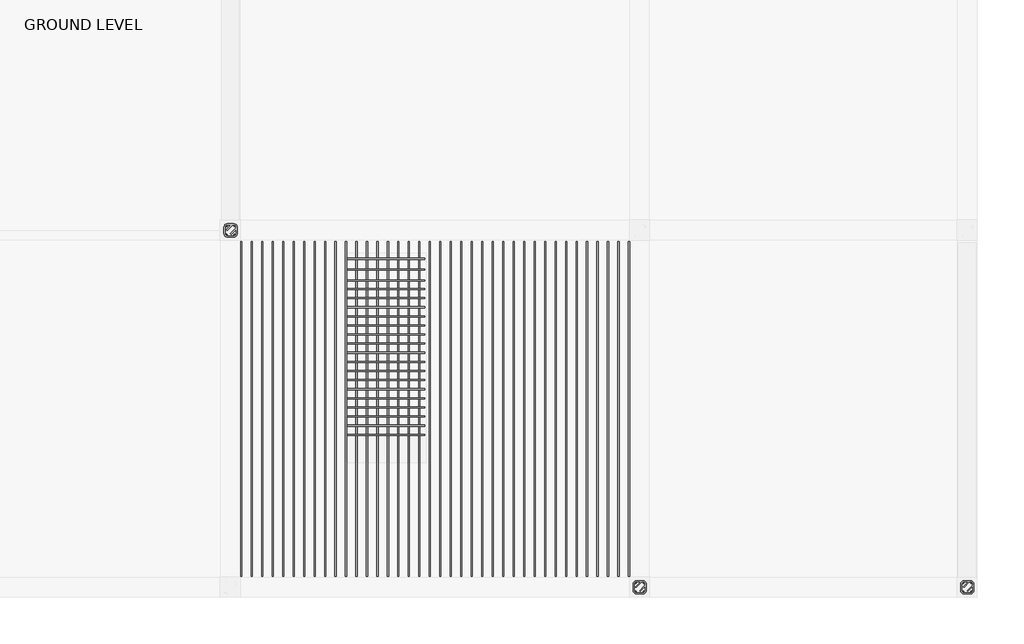
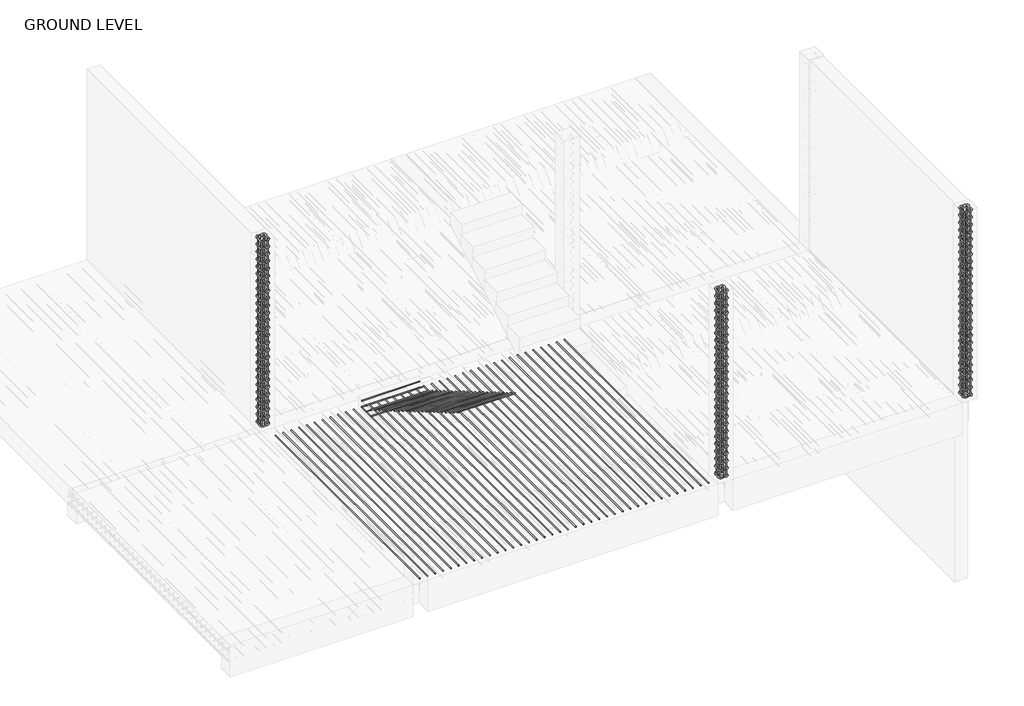
# One storey, part 4 of 8: 13 reinforcing bars.
"""IFC4 building model written with IfcOpenShell, lengths in millimetres."""

from ifc_helpers import new_model, si_unit, point, frame, origin, place, context, project, spatial, polyline, circle_curve, trimmed, segment, composite_curve, source, transform, mapped, element, save
from ifc_brep_helpers import swept_disk

model = new_model("IFC4")

# Units and contexts
model_context = context("Model", 3, world=origin())
ifc_project = project(units=[si_unit("LENGTHUNIT", "METRE", prefix="MILLI")], contexts=[model_context])

# Site, building, storey
site = spatial("IfcSite", under=ifc_project)
building = spatial("IfcBuilding", under=site)
storey = spatial("IfcBuildingStorey", under=building, Name="GROUND LEVEL", Elevation=0.0)

# Reinforcing bars
placement = place(None, origin())
reinforcing_bar_shape = source(origin(), model_context, "Body", "SolidModel", [
    swept_disk(composite_curve([segment(polyline([(-7435.1173382, -4134.0810507, -120.830741), (-7435.1173382, -358.1289151, -120.830741)]), True, "CONTINUOUS")], self_intersect=False), 6.35),
])
element("IfcReinforcingBar", 1, at=placement, inside=storey, context=model_context, shape_type="MappedRepresentation", body=[
    mapped(reinforcing_bar_shape, transform((0.0, 0.0, 0.0), x_axis=(1.0, 0.0, 0.0), y_axis=(0.0, 1.0, 0.0), z_axis=(0.0, 0.0, 1.0))),
    mapped(reinforcing_bar_shape, transform((-118.1294146, 0.0, 0.0), x_axis=(1.0, 0.0, 0.0), y_axis=(0.0, 1.0, 0.0), z_axis=(0.0, 0.0, 1.0))),
    mapped(reinforcing_bar_shape, transform((-236.2588293, 0.0, 0.0), x_axis=(1.0, 0.0, 0.0), y_axis=(0.0, 1.0, 0.0), z_axis=(0.0, 0.0, 1.0))),
    mapped(reinforcing_bar_shape, transform((-354.3882439, 0.0, 0.0), x_axis=(1.0, 0.0, 0.0), y_axis=(0.0, 1.0, 0.0), z_axis=(0.0, 0.0, 1.0))),
    mapped(reinforcing_bar_shape, transform((-472.5176586, 0.0, 0.0), x_axis=(1.0, 0.0, 0.0), y_axis=(0.0, 1.0, 0.0), z_axis=(0.0, 0.0, 1.0))),
    mapped(reinforcing_bar_shape, transform((-590.6470732, 0.0, 0.0), x_axis=(1.0, 0.0, 0.0), y_axis=(0.0, 1.0, 0.0), z_axis=(0.0, 0.0, 1.0))),
    mapped(reinforcing_bar_shape, transform((-708.7764878, 0.0, 0.0), x_axis=(1.0, 0.0, 0.0), y_axis=(0.0, 1.0, 0.0), z_axis=(0.0, 0.0, 1.0))),
    mapped(reinforcing_bar_shape, transform((-826.9059025, 0.0, 0.0), x_axis=(1.0, 0.0, 0.0), y_axis=(0.0, 1.0, 0.0), z_axis=(0.0, 0.0, 1.0))),
    mapped(reinforcing_bar_shape, transform((-945.0353171, 0.0, 0.0), x_axis=(1.0, 0.0, 0.0), y_axis=(0.0, 1.0, 0.0), z_axis=(0.0, 0.0, 1.0))),
    mapped(reinforcing_bar_shape, transform((-1063.1647318, 0.0, 0.0), x_axis=(1.0, 0.0, 0.0), y_axis=(0.0, 1.0, 0.0), z_axis=(0.0, 0.0, 1.0))),
    mapped(reinforcing_bar_shape, transform((-1181.2941464, 0.0, 0.0), x_axis=(1.0, 0.0, 0.0), y_axis=(0.0, 1.0, 0.0), z_axis=(0.0, 0.0, 1.0))),
    mapped(reinforcing_bar_shape, transform((-1299.423561, 0.0, 0.0), x_axis=(1.0, 0.0, 0.0), y_axis=(0.0, 1.0, 0.0), z_axis=(0.0, 0.0, 1.0))),
    mapped(reinforcing_bar_shape, transform((-1417.5529757, 0.0, 0.0), x_axis=(1.0, 0.0, 0.0), y_axis=(0.0, 1.0, 0.0), z_axis=(0.0, 0.0, 1.0))),
    mapped(reinforcing_bar_shape, transform((-1535.6823903, 0.0, 0.0), x_axis=(1.0, 0.0, 0.0), y_axis=(0.0, 1.0, 0.0), z_axis=(0.0, 0.0, 1.0))),
    mapped(reinforcing_bar_shape, transform((-1653.811805, 0.0, 0.0), x_axis=(1.0, 0.0, 0.0), y_axis=(0.0, 1.0, 0.0), z_axis=(0.0, 0.0, 1.0))),
    mapped(reinforcing_bar_shape, transform((-1771.9412196, 0.0, 0.0), x_axis=(1.0, 0.0, 0.0), y_axis=(0.0, 1.0, 0.0), z_axis=(0.0, 0.0, 1.0))),
    mapped(reinforcing_bar_shape, transform((-1890.0706342, 0.0, 0.0), x_axis=(1.0, 0.0, 0.0), y_axis=(0.0, 1.0, 0.0), z_axis=(0.0, 0.0, 1.0))),
    mapped(reinforcing_bar_shape, transform((-2008.2000489, 0.0, 0.0), x_axis=(1.0, 0.0, 0.0), y_axis=(0.0, 1.0, 0.0), z_axis=(0.0, 0.0, 1.0))),
    mapped(reinforcing_bar_shape, transform((-2126.3294635, 0.0, 0.0), x_axis=(1.0, 0.0, 0.0), y_axis=(0.0, 1.0, 0.0), z_axis=(0.0, 0.0, 1.0))),
    mapped(reinforcing_bar_shape, transform((-2244.4588782, 0.0, 0.0), x_axis=(1.0, 0.0, 0.0), y_axis=(0.0, 1.0, 0.0), z_axis=(0.0, 0.0, 1.0))),
    mapped(reinforcing_bar_shape, transform((-2362.5882928, 0.0, 0.0), x_axis=(1.0, 0.0, 0.0), y_axis=(0.0, 1.0, 0.0), z_axis=(0.0, 0.0, 1.0))),
    mapped(reinforcing_bar_shape, transform((-2480.7177075, 0.0, 0.0), x_axis=(1.0, 0.0, 0.0), y_axis=(0.0, 1.0, 0.0), z_axis=(0.0, 0.0, 1.0))),
    mapped(reinforcing_bar_shape, transform((-2598.8471221, 0.0, 0.0), x_axis=(1.0, 0.0, 0.0), y_axis=(0.0, 1.0, 0.0), z_axis=(0.0, 0.0, 1.0))),
    mapped(reinforcing_bar_shape, transform((-2716.9765367, 0.0, 0.0), x_axis=(1.0, 0.0, 0.0), y_axis=(0.0, 1.0, 0.0), z_axis=(0.0, 0.0, 1.0))),
    mapped(reinforcing_bar_shape, transform((-2835.1059514, 0.0, 0.0), x_axis=(1.0, 0.0, 0.0), y_axis=(0.0, 1.0, 0.0), z_axis=(0.0, 0.0, 1.0))),
    mapped(reinforcing_bar_shape, transform((-2953.235366, 0.0, 0.0), x_axis=(1.0, 0.0, 0.0), y_axis=(0.0, 1.0, 0.0), z_axis=(0.0, 0.0, 1.0))),
    mapped(reinforcing_bar_shape, transform((-3071.3647807, 0.0, 0.0), x_axis=(1.0, 0.0, 0.0), y_axis=(0.0, 1.0, 0.0), z_axis=(0.0, 0.0, 1.0))),
    mapped(reinforcing_bar_shape, transform((-3189.4941953, 0.0, 0.0), x_axis=(1.0, 0.0, 0.0), y_axis=(0.0, 1.0, 0.0), z_axis=(0.0, 0.0, 1.0))),
    mapped(reinforcing_bar_shape, transform((-3307.6236099, 0.0, 0.0), x_axis=(1.0, 0.0, 0.0), y_axis=(0.0, 1.0, 0.0), z_axis=(0.0, 0.0, 1.0))),
    mapped(reinforcing_bar_shape, transform((-3425.7530246, 0.0, 0.0), x_axis=(1.0, 0.0, 0.0), y_axis=(0.0, 1.0, 0.0), z_axis=(0.0, 0.0, 1.0))),
    mapped(reinforcing_bar_shape, transform((-3543.8824392, 0.0, 0.0), x_axis=(1.0, 0.0, 0.0), y_axis=(0.0, 1.0, 0.0), z_axis=(0.0, 0.0, 1.0))),
    mapped(reinforcing_bar_shape, transform((-3662.0118539, 0.0, 0.0), x_axis=(1.0, 0.0, 0.0), y_axis=(0.0, 1.0, 0.0), z_axis=(0.0, 0.0, 1.0))),
    mapped(reinforcing_bar_shape, transform((-3780.1412685, 0.0, 0.0), x_axis=(1.0, 0.0, 0.0), y_axis=(0.0, 1.0, 0.0), z_axis=(0.0, 0.0, 1.0))),
    mapped(reinforcing_bar_shape, transform((-3898.2706831, 0.0, 0.0), x_axis=(1.0, 0.0, 0.0), y_axis=(0.0, 1.0, 0.0), z_axis=(0.0, 0.0, 1.0))),
    mapped(reinforcing_bar_shape, transform((-4016.4000978, 0.0, 0.0), x_axis=(1.0, 0.0, 0.0), y_axis=(0.0, 1.0, 0.0), z_axis=(0.0, 0.0, 1.0))),
    mapped(reinforcing_bar_shape, transform((-4134.5295124, 0.0, 0.0), x_axis=(1.0, 0.0, 0.0), y_axis=(0.0, 1.0, 0.0), z_axis=(0.0, 0.0, 1.0))),
    mapped(reinforcing_bar_shape, transform((-4252.6589271, 0.0, 0.0), x_axis=(1.0, 0.0, 0.0), y_axis=(0.0, 1.0, 0.0), z_axis=(0.0, 0.0, 1.0))),
    mapped(reinforcing_bar_shape, transform((-4370.7883417, 0.0, 0.0), x_axis=(1.0, 0.0, 0.0), y_axis=(0.0, 1.0, 0.0), z_axis=(0.0, 0.0, 1.0))),
])
reinforcing_bar_2_shape = source(origin(), model_context, "Body", "SolidModel", [
    swept_disk(composite_curve([segment(polyline([(-7269.7123519, -4211.1006392, 3008.0), (-7269.7123519, -4211.1006392, 40.0)]), True, "CONTINUOUS")], self_intersect=False), 6.35),
])
element("IfcReinforcingBar", 2, at=placement, inside=storey, context=model_context, shape_type="MappedRepresentation", body=[
    mapped(reinforcing_bar_2_shape, transform((0.0, 0.0, 0.0), x_axis=(1.0, 0.0, 0.0), y_axis=(0.0, 1.0, 0.0), z_axis=(0.0, 0.0, 1.0))),
    mapped(reinforcing_bar_2_shape, transform((0.0, -96.9916148, 0.0), x_axis=(1.0, 0.0, 0.0), y_axis=(0.0, 1.0, 0.0), z_axis=(0.0, 0.0, 1.0))),
])
reinforcing_bar_3_shape = source(origin(), model_context, "Body", "SolidModel", [
    swept_disk(composite_curve([segment(polyline([(-7355.7786987, -4256.8741003, 3001.65), (-7300.0351358, -4201.1305373, 3001.65)]), True, "CONTINUOUS"), segment(trimmed(circle_curve(frame((-7277.8673382, -4223.2983349, 3001.65), z_axis=(0.0, 0.0, -1.0), x_axis=(-22.167797600000085, 22.167797600000085, 0.0)), 31.35), [point((-7300.0351358, -4201.1305373, 3001.65))], [point((-7246.5173382, -4223.2983349, 3001.65))], True, "CARTESIAN"), True, "CONTINUOUS"), segment(polyline([(-7246.5173382, -4223.2983349, 3001.65), (-7246.5173382, -4296.4983349, 3001.65)]), True, "CONTINUOUS"), segment(trimmed(circle_curve(frame((-7277.8673382, -4296.4983349, 3001.65), z_axis=(0.0, 0.0, -1.0), x_axis=(31.349999999999454, 0.0, 0.0)), 31.35), [point((-7246.5173382, -4296.4983349, 3001.65))], [point((-7277.8673382, -4327.8483349, 3001.65))], True, "CARTESIAN"), True, "CONTINUOUS"), segment(polyline([(-7277.8673382, -4327.8483349, 3001.65), (-7351.0673382, -4327.8483349, 3001.65)]), True, "CONTINUOUS"), segment(trimmed(circle_curve(frame((-7351.0673382, -4296.6343361, 3004.5669815), z_axis=(0.0, 0.09304566152621355, -0.9956618426308951), x_axis=(0.0, -31.2139987999999, -2.91698150000002)), 31.35), [point((-7351.0673382, -4327.8483349, 3001.65))], [point((-7382.4173382, -4296.6343361, 3004.5669815))], True, "CARTESIAN"), True, "CONTINUOUS"), segment(polyline([(-7382.4173382, -4296.6343361, 3004.5669815), (-7382.4173382, -4223.1623337, 3011.4330185)]), True, "CONTINUOUS"), segment(trimmed(circle_curve(frame((-7351.0673382, -4223.1623337, 3011.4330185), z_axis=(0.0, 0.09304566152621355, -0.9956618426308951), x_axis=(-31.349999999999454, 0.0, 0.0)), 31.35), [point((-7382.4173382, -4223.1623337, 3011.4330185))], [point((-7351.0673382, -4191.9483349, 3014.35))], True, "CARTESIAN"), True, "CONTINUOUS"), segment(polyline([(-7351.0673382, -4191.9483349, 3014.35), (-7277.8673382, -4191.9483349, 3014.35)]), True, "CONTINUOUS"), segment(trimmed(circle_curve(frame((-7277.8673382, -4223.2983349, 3014.35), z_axis=(0.0, 0.0, -1.0), x_axis=(0.0, 31.349999999999454, 0.0)), 31.35), [point((-7277.8673382, -4191.9483349, 3014.35))], [point((-7255.6995406, -4245.4661325, 3014.35))], True, "CARTESIAN"), True, "CONTINUOUS"), segment(polyline([(-7255.6995406, -4245.4661325, 3014.35), (-7311.4431035, -4301.2096954, 3014.35)]), True, "CONTINUOUS")], self_intersect=False), 6.35),
])
element("IfcReinforcingBar", 3, at=placement, inside=storey, context=model_context, shape_type="MappedRepresentation", body=[
    mapped(reinforcing_bar_3_shape, transform((0.0, 0.0, 0.0), x_axis=(1.0, 0.0, 0.0), y_axis=(0.0, 1.0, 0.0), z_axis=(0.0, 0.0, 1.0))),
    mapped(reinforcing_bar_3_shape, transform((0.0, 0.0, -118.212), x_axis=(1.0, 0.0, 0.0), y_axis=(0.0, 1.0, 0.0), z_axis=(0.0, 0.0, 1.0))),
    mapped(reinforcing_bar_3_shape, transform((0.0, 0.0, -236.424), x_axis=(1.0, 0.0, 0.0), y_axis=(0.0, 1.0, 0.0), z_axis=(0.0, 0.0, 1.0))),
    mapped(reinforcing_bar_3_shape, transform((0.0, 0.0, -354.636), x_axis=(1.0, 0.0, 0.0), y_axis=(0.0, 1.0, 0.0), z_axis=(0.0, 0.0, 1.0))),
    mapped(reinforcing_bar_3_shape, transform((0.0, 0.0, -472.848), x_axis=(1.0, 0.0, 0.0), y_axis=(0.0, 1.0, 0.0), z_axis=(0.0, 0.0, 1.0))),
    mapped(reinforcing_bar_3_shape, transform((0.0, 0.0, -591.06), x_axis=(1.0, 0.0, 0.0), y_axis=(0.0, 1.0, 0.0), z_axis=(0.0, 0.0, 1.0))),
    mapped(reinforcing_bar_3_shape, transform((0.0, 0.0, -709.272), x_axis=(1.0, 0.0, 0.0), y_axis=(0.0, 1.0, 0.0), z_axis=(0.0, 0.0, 1.0))),
    mapped(reinforcing_bar_3_shape, transform((0.0, 0.0, -827.484), x_axis=(1.0, 0.0, 0.0), y_axis=(0.0, 1.0, 0.0), z_axis=(0.0, 0.0, 1.0))),
    mapped(reinforcing_bar_3_shape, transform((0.0, 0.0, -945.696), x_axis=(1.0, 0.0, 0.0), y_axis=(0.0, 1.0, 0.0), z_axis=(0.0, 0.0, 1.0))),
    mapped(reinforcing_bar_3_shape, transform((0.0, 0.0, -1063.908), x_axis=(1.0, 0.0, 0.0), y_axis=(0.0, 1.0, 0.0), z_axis=(0.0, 0.0, 1.0))),
    mapped(reinforcing_bar_3_shape, transform((0.0, 0.0, -1182.12), x_axis=(1.0, 0.0, 0.0), y_axis=(0.0, 1.0, 0.0), z_axis=(0.0, 0.0, 1.0))),
    mapped(reinforcing_bar_3_shape, transform((0.0, 0.0, -1300.332), x_axis=(1.0, 0.0, 0.0), y_axis=(0.0, 1.0, 0.0), z_axis=(0.0, 0.0, 1.0))),
    mapped(reinforcing_bar_3_shape, transform((0.0, 0.0, -1418.544), x_axis=(1.0, 0.0, 0.0), y_axis=(0.0, 1.0, 0.0), z_axis=(0.0, 0.0, 1.0))),
    mapped(reinforcing_bar_3_shape, transform((0.0, 0.0, -1536.756), x_axis=(1.0, 0.0, 0.0), y_axis=(0.0, 1.0, 0.0), z_axis=(0.0, 0.0, 1.0))),
    mapped(reinforcing_bar_3_shape, transform((0.0, 0.0, -1654.968), x_axis=(1.0, 0.0, 0.0), y_axis=(0.0, 1.0, 0.0), z_axis=(0.0, 0.0, 1.0))),
    mapped(reinforcing_bar_3_shape, transform((0.0, 0.0, -1773.18), x_axis=(1.0, 0.0, 0.0), y_axis=(0.0, 1.0, 0.0), z_axis=(0.0, 0.0, 1.0))),
    mapped(reinforcing_bar_3_shape, transform((0.0, 0.0, -1891.392), x_axis=(1.0, 0.0, 0.0), y_axis=(0.0, 1.0, 0.0), z_axis=(0.0, 0.0, 1.0))),
    mapped(reinforcing_bar_3_shape, transform((0.0, 0.0, -2009.604), x_axis=(1.0, 0.0, 0.0), y_axis=(0.0, 1.0, 0.0), z_axis=(0.0, 0.0, 1.0))),
    mapped(reinforcing_bar_3_shape, transform((0.0, 0.0, -2127.816), x_axis=(1.0, 0.0, 0.0), y_axis=(0.0, 1.0, 0.0), z_axis=(0.0, 0.0, 1.0))),
    mapped(reinforcing_bar_3_shape, transform((0.0, 0.0, -2246.028), x_axis=(1.0, 0.0, 0.0), y_axis=(0.0, 1.0, 0.0), z_axis=(0.0, 0.0, 1.0))),
    mapped(reinforcing_bar_3_shape, transform((0.0, 0.0, -2364.24), x_axis=(1.0, 0.0, 0.0), y_axis=(0.0, 1.0, 0.0), z_axis=(0.0, 0.0, 1.0))),
    mapped(reinforcing_bar_3_shape, transform((0.0, 0.0, -2482.452), x_axis=(1.0, 0.0, 0.0), y_axis=(0.0, 1.0, 0.0), z_axis=(0.0, 0.0, 1.0))),
    mapped(reinforcing_bar_3_shape, transform((0.0, 0.0, -2600.664), x_axis=(1.0, 0.0, 0.0), y_axis=(0.0, 1.0, 0.0), z_axis=(0.0, 0.0, 1.0))),
    mapped(reinforcing_bar_3_shape, transform((0.0, 0.0, -2718.876), x_axis=(1.0, 0.0, 0.0), y_axis=(0.0, 1.0, 0.0), z_axis=(0.0, 0.0, 1.0))),
    mapped(reinforcing_bar_3_shape, transform((0.0, 0.0, -2837.088), x_axis=(1.0, 0.0, 0.0), y_axis=(0.0, 1.0, 0.0), z_axis=(0.0, 0.0, 1.0))),
    mapped(reinforcing_bar_3_shape, transform((0.0, 0.0, -2955.3), x_axis=(1.0, 0.0, 0.0), y_axis=(0.0, 1.0, 0.0), z_axis=(0.0, 0.0, 1.0))),
])
reinforcing_bar_4_shape = source(origin(), model_context, "Body", "SolidModel", [
    swept_disk(composite_curve([segment(polyline([(-7359.2223245, -4211.1006392, 3008.0), (-7359.2223245, -4211.1006392, 40.0)]), True, "CONTINUOUS")], self_intersect=False), 6.35),
])
element("IfcReinforcingBar", 4, at=placement, inside=storey, context=model_context, shape_type="MappedRepresentation", body=[
    mapped(reinforcing_bar_4_shape, transform((0.0, 0.0, 0.0), x_axis=(1.0, 0.0, 0.0), y_axis=(0.0, 1.0, 0.0), z_axis=(0.0, 0.0, 1.0))),
    mapped(reinforcing_bar_4_shape, transform((0.0, -96.9916148, 0.0), x_axis=(1.0, 0.0, 0.0), y_axis=(0.0, 1.0, 0.0), z_axis=(0.0, 0.0, 1.0))),
])
reinforcing_bar_5_shape = source(origin(), model_context, "Body", "SolidModel", [
    swept_disk(composite_curve([segment(polyline([(-3576.0006936, -4211.1006392, 3008.0), (-3576.0006936, -4211.1006392, 40.0)]), True, "CONTINUOUS")], self_intersect=False), 6.35),
])
element("IfcReinforcingBar", 5, at=placement, inside=storey, context=model_context, shape_type="MappedRepresentation", body=[
    mapped(reinforcing_bar_5_shape, transform((0.0, 0.0, 0.0), x_axis=(1.0, 0.0, 0.0), y_axis=(0.0, 1.0, 0.0), z_axis=(0.0, 0.0, 1.0))),
    mapped(reinforcing_bar_5_shape, transform((0.0, -96.9916148, 0.0), x_axis=(1.0, 0.0, 0.0), y_axis=(0.0, 1.0, 0.0), z_axis=(0.0, 0.0, 1.0))),
])
reinforcing_bar_6_shape = source(origin(), model_context, "Body", "SolidModel", [
    swept_disk(composite_curve([segment(polyline([(-3662.0670404, -4256.8741003, 3001.65), (-3606.3234775, -4201.1305373, 3001.65)]), True, "CONTINUOUS"), segment(trimmed(circle_curve(frame((-3584.1556799, -4223.2983349, 3001.65), z_axis=(0.0, 0.0, -1.0), x_axis=(-22.167797600000085, 22.167797600000085, 0.0)), 31.35), [point((-3606.3234775, -4201.1305373, 3001.65))], [point((-3552.8056799, -4223.2983349, 3001.65))], True, "CARTESIAN"), True, "CONTINUOUS"), segment(polyline([(-3552.8056799, -4223.2983349, 3001.65), (-3552.8056799, -4296.4983349, 3001.65)]), True, "CONTINUOUS"), segment(trimmed(circle_curve(frame((-3584.1556799, -4296.4983349, 3001.65), z_axis=(0.0, 0.0, -1.0), x_axis=(31.34999999999991, 0.0, 0.0)), 31.35), [point((-3552.8056799, -4296.4983349, 3001.65))], [point((-3584.1556799, -4327.8483349, 3001.65))], True, "CARTESIAN"), True, "CONTINUOUS"), segment(polyline([(-3584.1556799, -4327.8483349, 3001.65), (-3657.3556799, -4327.8483349, 3001.65)]), True, "CONTINUOUS"), segment(trimmed(circle_curve(frame((-3657.3556799, -4296.6343361, 3004.5669815), z_axis=(0.0, 0.09304566152621355, -0.9956618426308951), x_axis=(0.0, -31.2139987999999, -2.91698150000002)), 31.35), [point((-3657.3556799, -4327.8483349, 3001.65))], [point((-3688.7056799, -4296.6343361, 3004.5669815))], True, "CARTESIAN"), True, "CONTINUOUS"), segment(polyline([(-3688.7056799, -4296.6343361, 3004.5669815), (-3688.7056799, -4223.1623337, 3011.4330185)]), True, "CONTINUOUS"), segment(trimmed(circle_curve(frame((-3657.3556799, -4223.1623337, 3011.4330185), z_axis=(0.0, 0.09304566152621355, -0.9956618426308951), x_axis=(-31.350000000000364, 0.0, 0.0)), 31.35), [point((-3688.7056799, -4223.1623337, 3011.4330185))], [point((-3657.3556799, -4191.9483349, 3014.35))], True, "CARTESIAN"), True, "CONTINUOUS"), segment(polyline([(-3657.3556799, -4191.9483349, 3014.35), (-3584.1556799, -4191.9483349, 3014.35)]), True, "CONTINUOUS"), segment(trimmed(circle_curve(frame((-3584.1556799, -4223.2983349, 3014.35), z_axis=(0.0, 0.0, -1.0), x_axis=(0.0, 31.349999999999454, 0.0)), 31.35), [point((-3584.1556799, -4191.9483349, 3014.35))], [point((-3561.9878823, -4245.4661325, 3014.35))], True, "CARTESIAN"), True, "CONTINUOUS"), segment(polyline([(-3561.9878823, -4245.4661325, 3014.35), (-3617.7314452, -4301.2096954, 3014.35)]), True, "CONTINUOUS")], self_intersect=False), 6.35),
])
element("IfcReinforcingBar", 6, at=placement, inside=storey, context=model_context, shape_type="MappedRepresentation", body=[
    mapped(reinforcing_bar_6_shape, transform((0.0, 0.0, 0.0), x_axis=(1.0, 0.0, 0.0), y_axis=(0.0, 1.0, 0.0), z_axis=(0.0, 0.0, 1.0))),
    mapped(reinforcing_bar_6_shape, transform((0.0, 0.0, -118.212), x_axis=(1.0, 0.0, 0.0), y_axis=(0.0, 1.0, 0.0), z_axis=(0.0, 0.0, 1.0))),
    mapped(reinforcing_bar_6_shape, transform((0.0, 0.0, -236.424), x_axis=(1.0, 0.0, 0.0), y_axis=(0.0, 1.0, 0.0), z_axis=(0.0, 0.0, 1.0))),
    mapped(reinforcing_bar_6_shape, transform((0.0, 0.0, -354.636), x_axis=(1.0, 0.0, 0.0), y_axis=(0.0, 1.0, 0.0), z_axis=(0.0, 0.0, 1.0))),
    mapped(reinforcing_bar_6_shape, transform((0.0, 0.0, -472.848), x_axis=(1.0, 0.0, 0.0), y_axis=(0.0, 1.0, 0.0), z_axis=(0.0, 0.0, 1.0))),
    mapped(reinforcing_bar_6_shape, transform((0.0, 0.0, -591.06), x_axis=(1.0, 0.0, 0.0), y_axis=(0.0, 1.0, 0.0), z_axis=(0.0, 0.0, 1.0))),
    mapped(reinforcing_bar_6_shape, transform((0.0, 0.0, -709.272), x_axis=(1.0, 0.0, 0.0), y_axis=(0.0, 1.0, 0.0), z_axis=(0.0, 0.0, 1.0))),
    mapped(reinforcing_bar_6_shape, transform((0.0, 0.0, -827.484), x_axis=(1.0, 0.0, 0.0), y_axis=(0.0, 1.0, 0.0), z_axis=(0.0, 0.0, 1.0))),
    mapped(reinforcing_bar_6_shape, transform((0.0, 0.0, -945.696), x_axis=(1.0, 0.0, 0.0), y_axis=(0.0, 1.0, 0.0), z_axis=(0.0, 0.0, 1.0))),
    mapped(reinforcing_bar_6_shape, transform((0.0, 0.0, -1063.908), x_axis=(1.0, 0.0, 0.0), y_axis=(0.0, 1.0, 0.0), z_axis=(0.0, 0.0, 1.0))),
    mapped(reinforcing_bar_6_shape, transform((0.0, 0.0, -1182.12), x_axis=(1.0, 0.0, 0.0), y_axis=(0.0, 1.0, 0.0), z_axis=(0.0, 0.0, 1.0))),
    mapped(reinforcing_bar_6_shape, transform((0.0, 0.0, -1300.332), x_axis=(1.0, 0.0, 0.0), y_axis=(0.0, 1.0, 0.0), z_axis=(0.0, 0.0, 1.0))),
    mapped(reinforcing_bar_6_shape, transform((0.0, 0.0, -1418.544), x_axis=(1.0, 0.0, 0.0), y_axis=(0.0, 1.0, 0.0), z_axis=(0.0, 0.0, 1.0))),
    mapped(reinforcing_bar_6_shape, transform((0.0, 0.0, -1536.756), x_axis=(1.0, 0.0, 0.0), y_axis=(0.0, 1.0, 0.0), z_axis=(0.0, 0.0, 1.0))),
    mapped(reinforcing_bar_6_shape, transform((0.0, 0.0, -1654.968), x_axis=(1.0, 0.0, 0.0), y_axis=(0.0, 1.0, 0.0), z_axis=(0.0, 0.0, 1.0))),
    mapped(reinforcing_bar_6_shape, transform((0.0, 0.0, -1773.18), x_axis=(1.0, 0.0, 0.0), y_axis=(0.0, 1.0, 0.0), z_axis=(0.0, 0.0, 1.0))),
    mapped(reinforcing_bar_6_shape, transform((0.0, 0.0, -1891.392), x_axis=(1.0, 0.0, 0.0), y_axis=(0.0, 1.0, 0.0), z_axis=(0.0, 0.0, 1.0))),
    mapped(reinforcing_bar_6_shape, transform((0.0, 0.0, -2009.604), x_axis=(1.0, 0.0, 0.0), y_axis=(0.0, 1.0, 0.0), z_axis=(0.0, 0.0, 1.0))),
    mapped(reinforcing_bar_6_shape, transform((0.0, 0.0, -2127.816), x_axis=(1.0, 0.0, 0.0), y_axis=(0.0, 1.0, 0.0), z_axis=(0.0, 0.0, 1.0))),
    mapped(reinforcing_bar_6_shape, transform((0.0, 0.0, -2246.028), x_axis=(1.0, 0.0, 0.0), y_axis=(0.0, 1.0, 0.0), z_axis=(0.0, 0.0, 1.0))),
    mapped(reinforcing_bar_6_shape, transform((0.0, 0.0, -2364.24), x_axis=(1.0, 0.0, 0.0), y_axis=(0.0, 1.0, 0.0), z_axis=(0.0, 0.0, 1.0))),
    mapped(reinforcing_bar_6_shape, transform((0.0, 0.0, -2482.452), x_axis=(1.0, 0.0, 0.0), y_axis=(0.0, 1.0, 0.0), z_axis=(0.0, 0.0, 1.0))),
    mapped(reinforcing_bar_6_shape, transform((0.0, 0.0, -2600.664), x_axis=(1.0, 0.0, 0.0), y_axis=(0.0, 1.0, 0.0), z_axis=(0.0, 0.0, 1.0))),
    mapped(reinforcing_bar_6_shape, transform((0.0, 0.0, -2718.876), x_axis=(1.0, 0.0, 0.0), y_axis=(0.0, 1.0, 0.0), z_axis=(0.0, 0.0, 1.0))),
    mapped(reinforcing_bar_6_shape, transform((0.0, 0.0, -2837.088), x_axis=(1.0, 0.0, 0.0), y_axis=(0.0, 1.0, 0.0), z_axis=(0.0, 0.0, 1.0))),
    mapped(reinforcing_bar_6_shape, transform((0.0, 0.0, -2955.3), x_axis=(1.0, 0.0, 0.0), y_axis=(0.0, 1.0, 0.0), z_axis=(0.0, 0.0, 1.0))),
])
reinforcing_bar_7_shape = source(origin(), model_context, "Body", "SolidModel", [
    swept_disk(composite_curve([segment(polyline([(-3665.5106662, -4211.1006392, 3008.0), (-3665.5106662, -4211.1006392, 40.0)]), True, "CONTINUOUS")], self_intersect=False), 6.35),
])
element("IfcReinforcingBar", 7, at=placement, inside=storey, context=model_context, shape_type="MappedRepresentation", body=[
    mapped(reinforcing_bar_7_shape, transform((0.0, 0.0, 0.0), x_axis=(1.0, 0.0, 0.0), y_axis=(0.0, 1.0, 0.0), z_axis=(0.0, 0.0, 1.0))),
    mapped(reinforcing_bar_7_shape, transform((0.0, -96.9916148, 0.0), x_axis=(1.0, 0.0, 0.0), y_axis=(0.0, 1.0, 0.0), z_axis=(0.0, 0.0, 1.0))),
])
reinforcing_bar_8_shape = source(origin(), model_context, "Body", "SolidModel", [
    swept_disk(composite_curve([segment(polyline([(-11881.8006936, -183.9048321, 3008.0), (-11881.8006936, -183.9048321, 40.0)]), True, "CONTINUOUS")], self_intersect=False), 6.35),
])
element("IfcReinforcingBar", 8, at=placement, inside=storey, context=model_context, shape_type="MappedRepresentation", body=[
    mapped(reinforcing_bar_8_shape, transform((0.0, 0.0, 0.0), x_axis=(1.0, 0.0, 0.0), y_axis=(0.0, 1.0, 0.0), z_axis=(0.0, 0.0, 1.0))),
    mapped(reinforcing_bar_8_shape, transform((0.0, -96.9916148, 0.0), x_axis=(1.0, 0.0, 0.0), y_axis=(0.0, 1.0, 0.0), z_axis=(0.0, 0.0, 1.0))),
])
reinforcing_bar_9_shape = source(origin(), model_context, "Body", "SolidModel", [
    swept_disk(composite_curve([segment(polyline([(-11967.8670404, -229.6782932, 3001.65), (-11912.1234775, -173.9347303, 3001.65)]), True, "CONTINUOUS"), segment(trimmed(circle_curve(frame((-11889.9556799, -196.1025279, 3001.65), z_axis=(0.0, 0.0, -1.0), x_axis=(-22.167797599999176, 22.1677976, 0.0)), 31.35), [point((-11912.1234775, -173.9347303, 3001.65))], [point((-11858.6056799, -196.1025279, 3001.65))], True, "CARTESIAN"), True, "CONTINUOUS"), segment(polyline([(-11858.6056799, -196.1025279, 3001.65), (-11858.6056799, -269.3025279, 3001.65)]), True, "CONTINUOUS"), segment(trimmed(circle_curve(frame((-11889.9556799, -269.3025279, 3001.65), z_axis=(0.0, 0.0, -1.0), x_axis=(31.350000000000364, 0.0, 0.0)), 31.35), [point((-11858.6056799, -269.3025279, 3001.65))], [point((-11889.9556799, -300.6525279, 3001.65))], True, "CARTESIAN"), True, "CONTINUOUS"), segment(polyline([(-11889.9556799, -300.6525279, 3001.65), (-11963.1556799, -300.6525279, 3001.65)]), True, "CONTINUOUS"), segment(trimmed(circle_curve(frame((-11963.1556799, -269.4385291, 3004.5669815), z_axis=(0.0, 0.09304566152621355, -0.9956618426308951), x_axis=(0.0, -31.213998800000013, -2.91698150000002)), 31.35), [point((-11963.1556799, -300.6525279, 3001.65))], [point((-11994.5056799, -269.4385291, 3004.5669815))], True, "CARTESIAN"), True, "CONTINUOUS"), segment(polyline([(-11994.5056799, -269.4385291, 3004.5669815), (-11994.5056799, -195.9665266, 3011.4330185)]), True, "CONTINUOUS"), segment(trimmed(circle_curve(frame((-11963.1556799, -195.9665266, 3011.4330185), z_axis=(0.0, 0.09304566152621355, -0.9956618426308951), x_axis=(-31.349999999998545, 0.0, 0.0)), 31.35), [point((-11994.5056799, -195.9665266, 3011.4330185))], [point((-11963.1556799, -164.7525279, 3014.35))], True, "CARTESIAN"), True, "CONTINUOUS"), segment(polyline([(-11963.1556799, -164.7525279, 3014.35), (-11889.9556799, -164.7525279, 3014.35)]), True, "CONTINUOUS"), segment(trimmed(circle_curve(frame((-11889.9556799, -196.1025279, 3014.35), z_axis=(0.0, 0.0, -1.0), x_axis=(0.0, 31.350000000000023, 0.0)), 31.35), [point((-11889.9556799, -164.7525279, 3014.35))], [point((-11867.7878823, -218.2703255, 3014.35))], True, "CARTESIAN"), True, "CONTINUOUS"), segment(polyline([(-11867.7878823, -218.2703255, 3014.35), (-11923.5314452, -274.0138884, 3014.35)]), True, "CONTINUOUS")], self_intersect=False), 6.35),
])
element("IfcReinforcingBar", 9, at=placement, inside=storey, context=model_context, shape_type="MappedRepresentation", body=[
    mapped(reinforcing_bar_9_shape, transform((0.0, 0.0, 0.0), x_axis=(1.0, 0.0, 0.0), y_axis=(0.0, 1.0, 0.0), z_axis=(0.0, 0.0, 1.0))),
    mapped(reinforcing_bar_9_shape, transform((0.0, 0.0, -118.212), x_axis=(1.0, 0.0, 0.0), y_axis=(0.0, 1.0, 0.0), z_axis=(0.0, 0.0, 1.0))),
    mapped(reinforcing_bar_9_shape, transform((0.0, 0.0, -236.424), x_axis=(1.0, 0.0, 0.0), y_axis=(0.0, 1.0, 0.0), z_axis=(0.0, 0.0, 1.0))),
    mapped(reinforcing_bar_9_shape, transform((0.0, 0.0, -354.636), x_axis=(1.0, 0.0, 0.0), y_axis=(0.0, 1.0, 0.0), z_axis=(0.0, 0.0, 1.0))),
    mapped(reinforcing_bar_9_shape, transform((0.0, 0.0, -472.848), x_axis=(1.0, 0.0, 0.0), y_axis=(0.0, 1.0, 0.0), z_axis=(0.0, 0.0, 1.0))),
    mapped(reinforcing_bar_9_shape, transform((0.0, 0.0, -591.06), x_axis=(1.0, 0.0, 0.0), y_axis=(0.0, 1.0, 0.0), z_axis=(0.0, 0.0, 1.0))),
    mapped(reinforcing_bar_9_shape, transform((0.0, 0.0, -709.272), x_axis=(1.0, 0.0, 0.0), y_axis=(0.0, 1.0, 0.0), z_axis=(0.0, 0.0, 1.0))),
    mapped(reinforcing_bar_9_shape, transform((0.0, 0.0, -827.484), x_axis=(1.0, 0.0, 0.0), y_axis=(0.0, 1.0, 0.0), z_axis=(0.0, 0.0, 1.0))),
    mapped(reinforcing_bar_9_shape, transform((0.0, 0.0, -945.696), x_axis=(1.0, 0.0, 0.0), y_axis=(0.0, 1.0, 0.0), z_axis=(0.0, 0.0, 1.0))),
    mapped(reinforcing_bar_9_shape, transform((0.0, 0.0, -1063.908), x_axis=(1.0, 0.0, 0.0), y_axis=(0.0, 1.0, 0.0), z_axis=(0.0, 0.0, 1.0))),
    mapped(reinforcing_bar_9_shape, transform((0.0, 0.0, -1182.12), x_axis=(1.0, 0.0, 0.0), y_axis=(0.0, 1.0, 0.0), z_axis=(0.0, 0.0, 1.0))),
    mapped(reinforcing_bar_9_shape, transform((0.0, 0.0, -1300.332), x_axis=(1.0, 0.0, 0.0), y_axis=(0.0, 1.0, 0.0), z_axis=(0.0, 0.0, 1.0))),
    mapped(reinforcing_bar_9_shape, transform((0.0, 0.0, -1418.544), x_axis=(1.0, 0.0, 0.0), y_axis=(0.0, 1.0, 0.0), z_axis=(0.0, 0.0, 1.0))),
    mapped(reinforcing_bar_9_shape, transform((0.0, 0.0, -1536.756), x_axis=(1.0, 0.0, 0.0), y_axis=(0.0, 1.0, 0.0), z_axis=(0.0, 0.0, 1.0))),
    mapped(reinforcing_bar_9_shape, transform((0.0, 0.0, -1654.968), x_axis=(1.0, 0.0, 0.0), y_axis=(0.0, 1.0, 0.0), z_axis=(0.0, 0.0, 1.0))),
    mapped(reinforcing_bar_9_shape, transform((0.0, 0.0, -1773.18), x_axis=(1.0, 0.0, 0.0), y_axis=(0.0, 1.0, 0.0), z_axis=(0.0, 0.0, 1.0))),
    mapped(reinforcing_bar_9_shape, transform((0.0, 0.0, -1891.392), x_axis=(1.0, 0.0, 0.0), y_axis=(0.0, 1.0, 0.0), z_axis=(0.0, 0.0, 1.0))),
    mapped(reinforcing_bar_9_shape, transform((0.0, 0.0, -2009.604), x_axis=(1.0, 0.0, 0.0), y_axis=(0.0, 1.0, 0.0), z_axis=(0.0, 0.0, 1.0))),
    mapped(reinforcing_bar_9_shape, transform((0.0, 0.0, -2127.816), x_axis=(1.0, 0.0, 0.0), y_axis=(0.0, 1.0, 0.0), z_axis=(0.0, 0.0, 1.0))),
    mapped(reinforcing_bar_9_shape, transform((0.0, 0.0, -2246.028), x_axis=(1.0, 0.0, 0.0), y_axis=(0.0, 1.0, 0.0), z_axis=(0.0, 0.0, 1.0))),
    mapped(reinforcing_bar_9_shape, transform((0.0, 0.0, -2364.24), x_axis=(1.0, 0.0, 0.0), y_axis=(0.0, 1.0, 0.0), z_axis=(0.0, 0.0, 1.0))),
    mapped(reinforcing_bar_9_shape, transform((0.0, 0.0, -2482.452), x_axis=(1.0, 0.0, 0.0), y_axis=(0.0, 1.0, 0.0), z_axis=(0.0, 0.0, 1.0))),
    mapped(reinforcing_bar_9_shape, transform((0.0, 0.0, -2600.664), x_axis=(1.0, 0.0, 0.0), y_axis=(0.0, 1.0, 0.0), z_axis=(0.0, 0.0, 1.0))),
    mapped(reinforcing_bar_9_shape, transform((0.0, 0.0, -2718.876), x_axis=(1.0, 0.0, 0.0), y_axis=(0.0, 1.0, 0.0), z_axis=(0.0, 0.0, 1.0))),
    mapped(reinforcing_bar_9_shape, transform((0.0, 0.0, -2837.088), x_axis=(1.0, 0.0, 0.0), y_axis=(0.0, 1.0, 0.0), z_axis=(0.0, 0.0, 1.0))),
    mapped(reinforcing_bar_9_shape, transform((0.0, 0.0, -2955.3), x_axis=(1.0, 0.0, 0.0), y_axis=(0.0, 1.0, 0.0), z_axis=(0.0, 0.0, 1.0))),
])
reinforcing_bar_10_shape = source(origin(), model_context, "Body", "SolidModel", [
    swept_disk(composite_curve([segment(polyline([(-11971.3106662, -183.9048321, 3008.0), (-11971.3106662, -183.9048321, 40.0)]), True, "CONTINUOUS")], self_intersect=False), 6.35),
])
element("IfcReinforcingBar", 10, at=placement, inside=storey, context=model_context, shape_type="MappedRepresentation", body=[
    mapped(reinforcing_bar_10_shape, transform((0.0, 0.0, 0.0), x_axis=(1.0, 0.0, 0.0), y_axis=(0.0, 1.0, 0.0), z_axis=(0.0, 0.0, 1.0))),
    mapped(reinforcing_bar_10_shape, transform((0.0, -96.9916148, 0.0), x_axis=(1.0, 0.0, 0.0), y_axis=(0.0, 1.0, 0.0), z_axis=(0.0, 0.0, 1.0))),
])
reinforcing_bar_11_shape = source(origin(), model_context, "Body", "SolidModel", [
    swept_disk(composite_curve([segment(polyline([(-9739.1476583, -553.8305693, 36.435057), (-10613.5476583, -553.8305693, 36.435057)]), True, "CONTINUOUS")], self_intersect=False), 6.35),
])
element("IfcReinforcingBar", 11, at=placement, inside=storey, context=model_context, shape_type="MappedRepresentation", body=[
    mapped(reinforcing_bar_11_shape, transform((0.0, 0.0, 0.0), x_axis=(1.0, 0.0, 0.0), y_axis=(0.0, 1.0, 0.0), z_axis=(0.0, 0.0, 1.0))),
    mapped(reinforcing_bar_11_shape, transform((0.0, -121.7261241, 0.0), x_axis=(1.0, 0.0, 0.0), y_axis=(0.0, 1.0, 0.0), z_axis=(0.0, 0.0, 1.0))),
    mapped(reinforcing_bar_11_shape, transform((0.0, -243.4522481, 0.0), x_axis=(1.0, 0.0, 0.0), y_axis=(0.0, 1.0, 0.0), z_axis=(0.0, 0.0, 1.0))),
])
reinforcing_bar_12_shape = source(origin(), model_context, "Body", "SolidModel", [
    swept_disk(composite_curve([segment(polyline([(-9739.1476583, -553.8305693, 136.435057), (-10613.5476583, -553.8305693, 136.435057)]), True, "CONTINUOUS")], self_intersect=False), 6.35),
])
element("IfcReinforcingBar", 12, at=placement, inside=storey, context=model_context, shape_type="MappedRepresentation", body=[
    mapped(reinforcing_bar_12_shape, transform((0.0, 0.0, 0.0), x_axis=(1.0, 0.0, 0.0), y_axis=(0.0, 1.0, 0.0), z_axis=(0.0, 0.0, 1.0))),
    mapped(reinforcing_bar_12_shape, transform((0.0, -121.7261241, 0.0), x_axis=(1.0, 0.0, 0.0), y_axis=(0.0, 1.0, 0.0), z_axis=(0.0, 0.0, 1.0))),
    mapped(reinforcing_bar_12_shape, transform((0.0, -243.4522481, 0.0), x_axis=(1.0, 0.0, 0.0), y_axis=(0.0, 1.0, 0.0), z_axis=(0.0, 0.0, 1.0))),
])
reinforcing_bar_13_shape = source(origin(), model_context, "Body", "SolidModel", [
    swept_disk(composite_curve([segment(polyline([(-9739.1476583, -894.130393, 192.95667), (-10613.5476583, -894.130393, 192.95667)]), True, "CONTINUOUS")], self_intersect=False), 6.35),
])
element("IfcReinforcingBar", 13, at=placement, inside=storey, context=model_context, shape_type="MappedRepresentation", body=[
    mapped(reinforcing_bar_13_shape, transform((0.0, 0.0, 0.0), x_axis=(1.0, 0.0, 0.0), y_axis=(0.0, 1.0, 0.0), z_axis=(0.0, 0.0, 1.0))),
    mapped(reinforcing_bar_13_shape, transform((0.0, -102.7683285, 60.4519579), x_axis=(1.0, 0.0, 0.0), y_axis=(0.0, 1.0, 0.0), z_axis=(0.0, 0.0, 1.0))),
    mapped(reinforcing_bar_13_shape, transform((0.0, -205.536657, 120.9039159), x_axis=(1.0, 0.0, 0.0), y_axis=(0.0, 1.0, 0.0), z_axis=(0.0, 0.0, 1.0))),
    mapped(reinforcing_bar_13_shape, transform((0.0, -308.3049855, 181.3558738), x_axis=(1.0, 0.0, 0.0), y_axis=(0.0, 1.0, 0.0), z_axis=(0.0, 0.0, 1.0))),
    mapped(reinforcing_bar_13_shape, transform((0.0, -411.073314, 241.8078318), x_axis=(1.0, 0.0, 0.0), y_axis=(0.0, 1.0, 0.0), z_axis=(0.0, 0.0, 1.0))),
    mapped(reinforcing_bar_13_shape, transform((0.0, -513.8416425, 302.2597897), x_axis=(1.0, 0.0, 0.0), y_axis=(0.0, 1.0, 0.0), z_axis=(0.0, 0.0, 1.0))),
    mapped(reinforcing_bar_13_shape, transform((0.0, -616.609971, 362.7117476), x_axis=(1.0, 0.0, 0.0), y_axis=(0.0, 1.0, 0.0), z_axis=(0.0, 0.0, 1.0))),
    mapped(reinforcing_bar_13_shape, transform((0.0, -719.3782995, 423.1637056), x_axis=(1.0, 0.0, 0.0), y_axis=(0.0, 1.0, 0.0), z_axis=(0.0, 0.0, 1.0))),
    mapped(reinforcing_bar_13_shape, transform((0.0, -822.146628, 483.6156635), x_axis=(1.0, 0.0, 0.0), y_axis=(0.0, 1.0, 0.0), z_axis=(0.0, 0.0, 1.0))),
    mapped(reinforcing_bar_13_shape, transform((0.0, -924.9149565, 544.0676215), x_axis=(1.0, 0.0, 0.0), y_axis=(0.0, 1.0, 0.0), z_axis=(0.0, 0.0, 1.0))),
    mapped(reinforcing_bar_13_shape, transform((0.0, -1027.683285, 604.5195794), x_axis=(1.0, 0.0, 0.0), y_axis=(0.0, 1.0, 0.0), z_axis=(0.0, 0.0, 1.0))),
    mapped(reinforcing_bar_13_shape, transform((0.0, -1130.4516135, 664.9715373), x_axis=(1.0, 0.0, 0.0), y_axis=(0.0, 1.0, 0.0), z_axis=(0.0, 0.0, 1.0))),
    mapped(reinforcing_bar_13_shape, transform((0.0, -1233.219942, 725.4234953), x_axis=(1.0, 0.0, 0.0), y_axis=(0.0, 1.0, 0.0), z_axis=(0.0, 0.0, 1.0))),
    mapped(reinforcing_bar_13_shape, transform((0.0, -1335.9882705, 785.8754532), x_axis=(1.0, 0.0, 0.0), y_axis=(0.0, 1.0, 0.0), z_axis=(0.0, 0.0, 1.0))),
    mapped(reinforcing_bar_13_shape, transform((0.0, -1438.756599, 846.3274112), x_axis=(1.0, 0.0, 0.0), y_axis=(0.0, 1.0, 0.0), z_axis=(0.0, 0.0, 1.0))),
    mapped(reinforcing_bar_13_shape, transform((0.0, -1541.5249275, 906.7793691), x_axis=(1.0, 0.0, 0.0), y_axis=(0.0, 1.0, 0.0), z_axis=(0.0, 0.0, 1.0))),
    mapped(reinforcing_bar_13_shape, transform((0.0, -1644.293256, 967.231327), x_axis=(1.0, 0.0, 0.0), y_axis=(0.0, 1.0, 0.0), z_axis=(0.0, 0.0, 1.0))),
    mapped(reinforcing_bar_13_shape, transform((0.0, -1747.0615845, 1027.683285), x_axis=(1.0, 0.0, 0.0), y_axis=(0.0, 1.0, 0.0), z_axis=(0.0, 0.0, 1.0))),
    mapped(reinforcing_bar_13_shape, transform((0.0, -1849.829913, 1088.1352429), x_axis=(1.0, 0.0, 0.0), y_axis=(0.0, 1.0, 0.0), z_axis=(0.0, 0.0, 1.0))),
    mapped(reinforcing_bar_13_shape, transform((0.0, -1952.5982415, 1148.5872009), x_axis=(1.0, 0.0, 0.0), y_axis=(0.0, 1.0, 0.0), z_axis=(0.0, 0.0, 1.0))),
    mapped(reinforcing_bar_13_shape, transform((0.0, -2055.36657, 1209.0391588), x_axis=(1.0, 0.0, 0.0), y_axis=(0.0, 1.0, 0.0), z_axis=(0.0, 0.0, 1.0))),
    mapped(reinforcing_bar_13_shape, transform((0.0, -2158.1348985, 1269.4911167), x_axis=(1.0, 0.0, 0.0), y_axis=(0.0, 1.0, 0.0), z_axis=(0.0, 0.0, 1.0))),
])

save(model, "model.ifc")

# Revit data of these elements
# Elements 1, 2, 3, 4, 5, 6, 7, 8, 9, 10, 11, 12, 13 (IfcReinforcingBar)
#   Phase Created = New Construction
